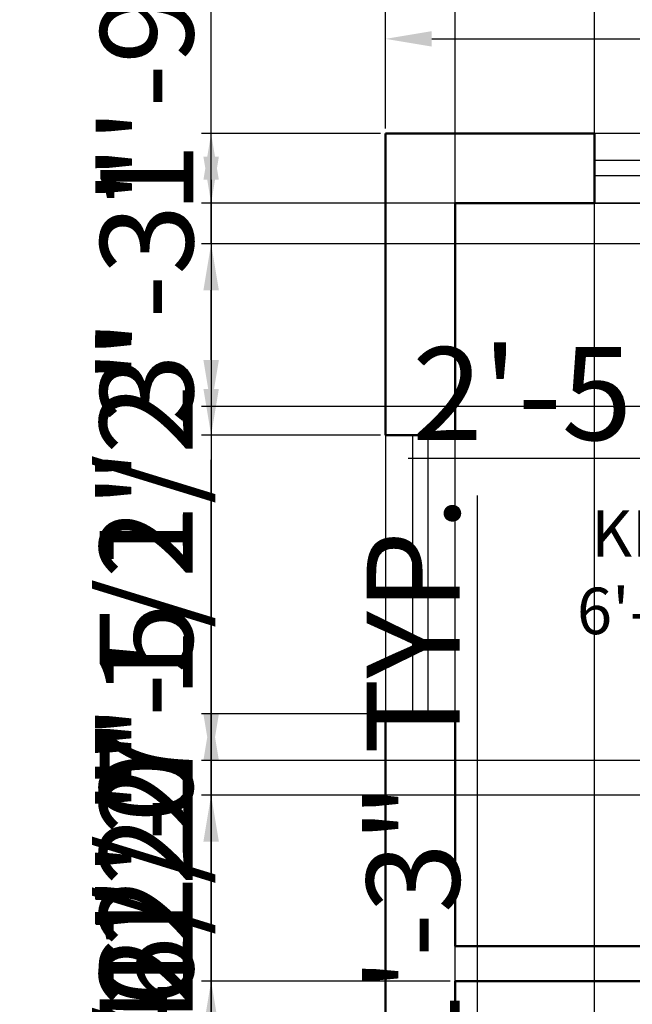
# Model space of a CAD drawing. Units: inches. Extents: x 1086 to 1501, y 383 to 973.
# Tile 4 of 7: x 1086 to 1165, y 723 to 850. Entities that reach past the tile are written whole.
import ezdxf

# ---------------------------------------------------------------- set-up
doc = ezdxf.new("R2010")
doc.units = ezdxf.units.IN
for name, color, linetype, lineweight in [('A-ANNO-DIMS', 2, 'Continuous', 18), ('A-AREA-IDEN', 7, 'Continuous', 25), ('wall', 7, 'Continuous', 50), ('window', 81, 'Continuous', 25)]:
    doc.layers.add(name, color=color, linetype=linetype, lineweight=lineweight)
doc.styles.get("Standard").update_dxf_attribs({"font": 'arial.ttf'})
doc.dimstyles.new('ISO-25', dxfattribs={"dimtxt": 12, "dimasz": 6, "dimexe": 1.25, "dimexo": 0.625, "dimtad": 1, "dimdec": 1, "dimlunit": 3, "dimtxsty": 'Standard', "dimcen": 2.5, "dimadec": 0, "dimazin": 0, "dimtfac": 1, "dimtdec": 1, "dimtmove": 0, "dimatfit": 3, "dimfxl": 1, "dimarcsym": 0})

# ---------------------------------------------------------------- blocks, each defined once
blk = doc.blocks.new('w1')
at = {"layer": 'window'}
for p, q in [((1475.33, 845.32), (1475.33, 809.32)), ((1477.33, 845.32), (1477.33, 809.32))]:
    blk.add_line(p, q, dxfattribs=at)
blk.add_lwpolyline([(1471.83, 809.32), (1480.83, 809.32), (1480.83, 845.32), (1471.83, 845.32)], close=True, dxfattribs=at)
blk = doc.blocks.new('*D9')
at = {"layer": 'A-ANNO-DIMS', "color": 0, "lineweight": -2, "transparency": 16777216}
for p, q in [((1133.43, 835.83), (1133.43, 848.67)), ((1403.43, 835.83), (1403.43, 848.67)), ((1139.43, 847.42), (1397.43, 847.42))]:
    blk.add_line(p, q, dxfattribs=at)
at = {"layer": 'A-ANNO-DIMS', "color": 0, "transparency": 16777216}
for points in [[(1139.43, 848.42), (1139.43, 846.42), (1133.43, 847.42)], [(1397.43, 848.42), (1397.43, 846.42), (1403.43, 847.42)]]:
    blk.add_solid(points, dxfattribs=at)
at = {"layer": 'Defpoints', "color": 0, "transparency": 16777216}
for p in [(1403.43, 847.42), (1133.43, 835.21), (1403.43, 835.21)]:
    blk.add_point(p, dxfattribs=at)
at = {"layer": 'A-ANNO-DIMS', "color": 0, "transparency": 16777216, "insert": (1268.43, 854.18), "char_height": 12, "attachment_point": 5}
blk.add_mtext('22\'-6"', dxfattribs=at)
blk = doc.blocks.new('*D18')
at = {"layer": 'A-ANNO-DIMS', "color": 0, "lineweight": -2, "transparency": 16777216}
for p, q in [((1244.93, 789.33), (1244.93, 794.46)), ((1274.43, 789.33), (1274.43, 794.46)), ((1244.93, 793.21), (1136.37, 793.21)), ((1268.43, 793.21), (1250.93, 793.21))]:
    blk.add_line(p, q, dxfattribs=at)
at = {"layer": 'A-ANNO-DIMS', "color": 0, "transparency": 16777216}
for points in [[(1250.93, 794.21), (1250.93, 792.21), (1244.93, 793.21)], [(1268.43, 794.21), (1268.43, 792.21), (1274.43, 793.21)]]:
    blk.add_solid(points, dxfattribs=at)
at = {"layer": 'Defpoints', "color": 0, "transparency": 16777216}
for p in [(1244.93, 793.21), (1244.93, 788.71), (1274.43, 788.71)]:
    blk.add_point(p, dxfattribs=at)
at = {"layer": 'A-ANNO-DIMS', "color": 0, "transparency": 16777216, "insert": (1187.65, 800.04), "char_height": 12, "attachment_point": 5}
blk.add_mtext('2\'-5 1/2" TYP.', dxfattribs=at)
blk = doc.blocks.new('*D25')
at = {"layer": 'A-ANNO-DIMS', "color": 0, "lineweight": -2, "transparency": 16777216}
for p, q in [((1147.7, 709.78), (1147.7, 712.78)), ((1163.51, 709.78), (1163.51, 712.78)), ((1153.7, 711.53), (1157.51, 711.53)), ((1163.51, 711.53), (1340.15, 711.53))]:
    blk.add_line(p, q, dxfattribs=at)
at = {"layer": 'A-ANNO-DIMS', "color": 0, "transparency": 16777216}
for points in [[(1153.7, 712.53), (1153.7, 710.53), (1147.7, 711.53)], [(1157.51, 712.53), (1157.51, 710.53), (1163.51, 711.53)]]:
    blk.add_solid(points, dxfattribs=at)
at = {"layer": 'Defpoints', "color": 0, "transparency": 16777216}
for p in [(1163.51, 711.53), (1147.7, 709.16), (1163.51, 709.16)]:
    blk.add_point(p, dxfattribs=at)
at = {"layer": 'A-ANNO-DIMS', "color": 0, "transparency": 16777216, "insert": (1254.83, 718.36), "char_height": 12, "attachment_point": 5}
blk.add_mtext('END CHAIR 1\'-4" TYP.', dxfattribs=at)
blk = doc.blocks.new('*D26')
at = {"layer": 'A-ANNO-DIMS', "color": 0, "lineweight": -2, "transparency": 16777216}
for p, q in [((1145.33, 709.16), (1145.33, 788.42)), ((1147.07, 709.16), (1144.08, 709.16)), ((1145.33, 700.13), (1145.33, 703.16)), ((1147.07, 694.13), (1144.08, 694.13))]:
    blk.add_line(p, q, dxfattribs=at)
at = {"layer": 'A-ANNO-DIMS', "color": 0, "transparency": 16777216}
for points in [[(1144.33, 703.16), (1146.33, 703.16), (1145.33, 709.16)], [(1144.33, 700.13), (1146.33, 700.13), (1145.33, 694.13)]]:
    blk.add_solid(points, dxfattribs=at)
at = {"layer": 'Defpoints', "color": 0, "transparency": 16777216}
for p in [(1145.33, 709.16), (1147.7, 709.16), (1147.7, 694.13)]:
    blk.add_point(p, dxfattribs=at)
at = {"layer": 'A-ANNO-DIMS', "color": 0, "transparency": 16777216, "insert": (1138.57, 751.79), "char_height": 12, "attachment_point": 5, "rotation": 90}
blk.add_mtext('1\'-3" TYP.', dxfattribs=at)
blk = doc.blocks.new('*D29')
at = {"layer": 'A-ANNO-DIMS', "color": 0, "lineweight": -2, "transparency": 16777216}
for p, q in [((1133.43, 835.83), (1133.43, 867.19)), ((1160.43, 835.83), (1160.43, 867.19)), ((1139.43, 865.94), (1154.43, 865.94)), ((1160.43, 865.94), (1199.78, 865.94))]:
    blk.add_line(p, q, dxfattribs=at)
at = {"layer": 'A-ANNO-DIMS', "color": 0, "transparency": 16777216}
for points in [[(1139.43, 866.94), (1139.43, 864.94), (1133.43, 865.94)], [(1154.43, 866.94), (1154.43, 864.94), (1160.43, 865.94)]]:
    blk.add_solid(points, dxfattribs=at)
at = {"layer": 'Defpoints', "color": 0, "transparency": 16777216}
for p in [(1160.43, 865.94), (1133.43, 835.21), (1160.43, 835.21)]:
    blk.add_point(p, dxfattribs=at)
at = {"layer": 'A-ANNO-DIMS', "color": 0, "transparency": 16777216, "insert": (1183.11, 872.7), "char_height": 12, "attachment_point": 5}
blk.add_mtext('2\'-3"', dxfattribs=at)
blk = doc.blocks.new('*D32')
at = {"layer": 'A-ANNO-DIMS', "color": 0, "lineweight": -2, "transparency": 16777216}
for p, q in [((1132.8, 835.21), (1109.68, 835.21)), ((1110.93, 829.21), (1110.93, 802.21)), ((1132.8, 796.21), (1109.68, 796.21))]:
    blk.add_line(p, q, dxfattribs=at)
at = {"layer": 'A-ANNO-DIMS', "color": 0, "transparency": 16777216}
for points in [[(1109.93, 829.21), (1111.93, 829.21), (1110.93, 835.21)], [(1109.93, 802.21), (1111.93, 802.21), (1110.93, 796.21)]]:
    blk.add_solid(points, dxfattribs=at)
at = {"layer": 'Defpoints', "color": 0, "transparency": 16777216}
for p in [(1133.43, 835.21), (1110.93, 796.21), (1133.43, 796.21)]:
    blk.add_point(p, dxfattribs=at)
at = {"layer": 'A-ANNO-DIMS', "color": 0, "transparency": 16777216, "insert": (1104.17, 815.71), "char_height": 12, "attachment_point": 5, "rotation": 90}
blk.add_mtext('3\'-3"', dxfattribs=at)
blk = doc.blocks.new('*D33')
at = {"layer": 'A-ANNO-DIMS', "color": 0, "lineweight": -2, "transparency": 16777216}
for p, q in [((1132.8, 760.21), (1109.68, 760.21)), ((1110.93, 754.21), (1110.93, 688.12)), ((1132.8, 682.12), (1109.68, 682.12))]:
    blk.add_line(p, q, dxfattribs=at)
at = {"layer": 'A-ANNO-DIMS', "color": 0, "transparency": 16777216}
for points in [[(1109.93, 754.21), (1111.93, 754.21), (1110.93, 760.21)], [(1109.93, 688.12), (1111.93, 688.12), (1110.93, 682.12)]]:
    blk.add_solid(points, dxfattribs=at)
at = {"layer": 'Defpoints', "color": 0, "transparency": 16777216}
for p in [(1133.43, 760.21), (1110.93, 682.12), (1133.43, 682.12)]:
    blk.add_point(p, dxfattribs=at)
at = {"layer": 'A-ANNO-DIMS', "color": 0, "transparency": 16777216, "insert": (1104.18, 721.16), "char_height": 12, "attachment_point": 5, "rotation": 90}
blk.add_mtext('6\'-6"', dxfattribs=at)
blk = doc.blocks.new('*D40')
at = {"layer": 'A-ANNO-DIMS', "color": 0, "lineweight": -2, "transparency": 16777216}
for p, q in [((1142.43, 502.33), (1142.43, 867.19)), ((1269.93, 502.33), (1269.93, 867.19)), ((1148.43, 865.94), (1263.93, 865.94))]:
    blk.add_line(p, q, dxfattribs=at)
at = {"layer": 'A-ANNO-DIMS', "color": 0, "transparency": 16777216}
for points in [[(1148.43, 866.94), (1148.43, 864.94), (1142.43, 865.94)], [(1263.93, 866.94), (1263.93, 864.94), (1269.93, 865.94)]]:
    blk.add_solid(points, dxfattribs=at)
at = {"layer": 'Defpoints', "color": 0, "transparency": 16777216}
for p in [(1269.93, 865.94), (1142.43, 501.71), (1269.93, 501.71)]:
    blk.add_point(p, dxfattribs=at)
at = {"layer": 'A-ANNO-DIMS', "color": 0, "transparency": 16777216, "insert": (1206.18, 872.77), "char_height": 12, "attachment_point": 5}
blk.add_mtext('10\'-7 1/2"', dxfattribs=at)
blk = doc.blocks.new('*D41')
at = {"layer": 'A-ANNO-DIMS', "color": 0, "lineweight": -2, "transparency": 16777216}
for p, q in [((1141.8, 725.71), (1109.68, 725.71)), ((1110.93, 507.71), (1110.93, 719.71)), ((1141.8, 501.71), (1109.68, 501.71))]:
    blk.add_line(p, q, dxfattribs=at)
at = {"layer": 'A-ANNO-DIMS', "color": 0, "transparency": 16777216}
for points in [[(1109.93, 719.71), (1111.93, 719.71), (1110.93, 725.71)], [(1109.93, 507.71), (1111.93, 507.71), (1110.93, 501.71)]]:
    blk.add_solid(points, dxfattribs=at)
at = {"layer": 'Defpoints', "color": 0, "transparency": 16777216}
for p in [(1110.93, 725.71), (1142.43, 725.71), (1142.43, 501.71)]:
    blk.add_point(p, dxfattribs=at)
at = {"layer": 'A-ANNO-DIMS', "color": 0, "transparency": 16777216, "insert": (1104.18, 613.71), "char_height": 12, "attachment_point": 5, "rotation": 90}
blk.add_mtext('18\'-8"', dxfattribs=at)
blk = doc.blocks.new('*D49')
at = {"layer": 'A-ANNO-DIMS', "color": 0, "lineweight": -2, "transparency": 16777216}
for p, q in [((1110.93, 760.21), (1110.93, 766.21)), ((1218.3, 754.21), (1109.68, 754.21)), ((1110.93, 754.21), (1110.93, 749.71)), ((1218.3, 749.71), (1109.68, 749.71)), ((1110.93, 743.71), (1110.93, 676.6))]:
    blk.add_line(p, q, dxfattribs=at)
at = {"layer": 'A-ANNO-DIMS', "color": 0, "transparency": 16777216}
for points in [[(1109.93, 760.21), (1111.93, 760.21), (1110.93, 754.21)], [(1109.93, 743.71), (1111.93, 743.71), (1110.93, 749.71)]]:
    blk.add_solid(points, dxfattribs=at)
at = {"layer": 'Defpoints', "color": 0, "transparency": 16777216}
for p in [(1218.93, 754.21), (1110.93, 749.71), (1218.93, 749.71)]:
    blk.add_point(p, dxfattribs=at)
at = {"layer": 'A-ANNO-DIMS', "color": 0, "transparency": 16777216, "insert": (1104.1, 707.15), "char_height": 12, "attachment_point": 5, "rotation": 90}
blk.add_mtext('0\'-4 1/2"', dxfattribs=at)
blk = doc.blocks.new('*D52')
at = {"layer": 'A-ANNO-DIMS', "color": 0, "lineweight": -2, "transparency": 16777216}
for p, q in [((1110.93, 692.71), (1110.93, 759.82)), ((1273.8, 686.71), (1109.68, 686.71)), ((1110.93, 682.21), (1110.93, 686.71)), ((1273.8, 682.21), (1109.68, 682.21)), ((1110.93, 676.21), (1110.93, 670.21))]:
    blk.add_line(p, q, dxfattribs=at)
at = {"layer": 'A-ANNO-DIMS', "color": 0, "transparency": 16777216}
for points in [[(1109.93, 692.71), (1111.93, 692.71), (1110.93, 686.71)], [(1109.93, 676.21), (1111.93, 676.21), (1110.93, 682.21)]]:
    blk.add_solid(points, dxfattribs=at)
at = {"layer": 'Defpoints', "color": 0, "transparency": 16777216}
for p in [(1110.93, 686.71), (1274.43, 686.71), (1274.43, 682.21)]:
    blk.add_point(p, dxfattribs=at)
at = {"layer": 'A-ANNO-DIMS', "color": 0, "transparency": 16777216, "insert": (1104.1, 729.26), "char_height": 12, "attachment_point": 5, "rotation": 90}
blk.add_mtext('0\'-4 1/2"', dxfattribs=at)
blk = doc.blocks.new('*D53')
at = {"layer": 'A-ANNO-DIMS', "color": 0, "lineweight": -2, "transparency": 16777216}
for p, q in [((1110.93, 686.71), (1110.93, 752.69)), ((1269.3, 686.71), (1109.68, 686.71)), ((1110.93, 679.21), (1110.93, 680.71)), ((1269.3, 673.21), (1109.68, 673.21))]:
    blk.add_line(p, q, dxfattribs=at)
at = {"layer": 'A-ANNO-DIMS', "color": 0, "transparency": 16777216}
for points in [[(1109.93, 680.71), (1111.93, 680.71), (1110.93, 686.71)], [(1109.93, 679.21), (1111.93, 679.21), (1110.93, 673.21)]]:
    blk.add_solid(points, dxfattribs=at)
at = {"layer": 'Defpoints', "color": 0, "transparency": 16777216}
for p in [(1110.93, 686.71), (1269.93, 686.71), (1269.93, 673.21)]:
    blk.add_point(p, dxfattribs=at)
at = {"layer": 'A-ANNO-DIMS', "color": 0, "transparency": 16777216, "insert": (1104.1, 722.7), "char_height": 12, "attachment_point": 5, "rotation": 90}
blk.add_mtext('1\'-1 1/2"', dxfattribs=at)
blk = doc.blocks.new('*D56')
at = {"layer": 'A-ANNO-DIMS', "color": 0, "lineweight": -2, "transparency": 16777216}
for p, q in [((1110.93, 832.21), (1110.93, 838.21)), ((1218.3, 826.21), (1109.68, 826.21)), ((1110.93, 826.21), (1110.93, 820.94)), ((1221.46, 820.94), (1109.68, 820.94)), ((1110.93, 814.94), (1110.93, 747.83))]:
    blk.add_line(p, q, dxfattribs=at)
at = {"layer": 'A-ANNO-DIMS', "color": 0, "transparency": 16777216}
for points in [[(1109.93, 832.21), (1111.93, 832.21), (1110.93, 826.21)], [(1109.93, 814.94), (1111.93, 814.94), (1110.93, 820.94)]]:
    blk.add_solid(points, dxfattribs=at)
at = {"layer": 'Defpoints', "color": 0, "transparency": 16777216}
for p in [(1218.93, 826.21), (1110.93, 820.94), (1222.08, 820.94)]:
    blk.add_point(p, dxfattribs=at)
at = {"layer": 'A-ANNO-DIMS', "color": 0, "transparency": 16777216, "insert": (1104.1, 778.39), "char_height": 12, "attachment_point": 5, "rotation": 90}
blk.add_mtext('0\'-5 1/2"', dxfattribs=at)
blk = doc.blocks.new('*D57')
at = {"layer": 'A-ANNO-DIMS', "color": 0, "lineweight": -2, "transparency": 16777216}
for p, q in [((1110.93, 820.94), (1110.93, 858.96)), ((1221.46, 820.94), (1109.68, 820.94)), ((1110.93, 805.94), (1110.93, 814.94)), ((1221.46, 799.94), (1109.68, 799.94))]:
    blk.add_line(p, q, dxfattribs=at)
at = {"layer": 'A-ANNO-DIMS', "color": 0, "transparency": 16777216}
for points in [[(1109.93, 814.94), (1111.93, 814.94), (1110.93, 820.94)], [(1109.93, 805.94), (1111.93, 805.94), (1110.93, 799.94)]]:
    blk.add_solid(points, dxfattribs=at)
at = {"layer": 'Defpoints', "color": 0, "transparency": 16777216}
for p in [(1110.93, 820.94), (1222.08, 820.94), (1222.08, 799.94)]:
    blk.add_point(p, dxfattribs=at)
at = {"layer": 'A-ANNO-DIMS', "color": 0, "transparency": 16777216, "insert": (1104.18, 842.95), "char_height": 12, "attachment_point": 5, "rotation": 90}
blk.add_mtext('1\'-9"', dxfattribs=at)
blk = doc.blocks.new('*D65')
at = {"layer": 'A-ANNO-DIMS', "color": 0, "lineweight": -2, "transparency": 16777216}
for p, q in [((1110.93, 725.71), (1110.93, 793.02)), ((1141.8, 725.71), (1109.68, 725.71)), ((1110.93, 700.13), (1110.93, 719.71)), ((1141.8, 694.13), (1109.68, 694.13))]:
    blk.add_line(p, q, dxfattribs=at)
at = {"layer": 'A-ANNO-DIMS', "color": 0, "transparency": 16777216}
for points in [[(1109.93, 719.71), (1111.93, 719.71), (1110.93, 725.71)], [(1109.93, 700.13), (1111.93, 700.13), (1110.93, 694.13)]]:
    blk.add_solid(points, dxfattribs=at)
at = {"layer": 'Defpoints', "color": 0, "transparency": 16777216}
for p in [(1110.93, 725.71), (1142.43, 725.71), (1142.43, 694.13)]:
    blk.add_point(p, dxfattribs=at)
at = {"layer": 'A-ANNO-DIMS', "color": 0, "transparency": 16777216, "insert": (1104.1, 762.36), "char_height": 12, "attachment_point": 5, "rotation": 90}
blk.add_mtext('2\'-7 1/2"', dxfattribs=at)
blk = doc.blocks.new('*D71')
at = {"layer": 'A-ANNO-DIMS', "color": 0, "lineweight": -2, "transparency": 16777216}
for p, q in [((1142.43, 589.29), (1142.43, 867.19)), ((1160.43, 589.29), (1160.43, 867.19)), ((1148.43, 865.94), (1154.43, 865.94)), ((1160.43, 865.94), (1198.45, 865.94))]:
    blk.add_line(p, q, dxfattribs=at)
at = {"layer": 'A-ANNO-DIMS', "color": 0, "transparency": 16777216}
for points in [[(1148.43, 866.94), (1148.43, 864.94), (1142.43, 865.94)], [(1154.43, 866.94), (1154.43, 864.94), (1160.43, 865.94)]]:
    blk.add_solid(points, dxfattribs=at)
at = {"layer": 'Defpoints', "color": 0, "transparency": 16777216}
for p in [(1160.43, 865.94), (1142.43, 588.67), (1160.43, 588.67)]:
    blk.add_point(p, dxfattribs=at)
at = {"layer": 'A-ANNO-DIMS', "color": 0, "transparency": 16777216, "insert": (1182.44, 872.69), "char_height": 12, "attachment_point": 5}
blk.add_mtext('1\'-6"', dxfattribs=at)

msp = doc.modelspace()

# ---------------------------------------------------------------- linework, layer by layer
at = {"layer": 'wall'}
for p, q in [((1133.43, 835.21), (1133.43, 796.21)), ((1160.43, 835.21), (1133.43, 835.21)), ((1160.43, 826.21), (1160.43, 835.21)), ((1142.43, 826.21), (1142.43, 796.21)), ((1160.43, 826.21), (1142.43, 826.21)), ((1142.43, 796.21), (1133.43, 796.21)), ((1142.43, 760.21), (1133.43, 760.21)), ((1133.43, 760.21), (1133.43, 682.12)), ((1142.43, 760.21), (1142.43, 730.21)), ((1214.43, 730.21), (1142.43, 730.21)), ((1218.93, 725.71), (1142.43, 725.71)), ((1142.43, 725.71), (1142.43, 682.12))]:
    msp.add_line(p, q, dxfattribs=at)

# ---------------------------------------------------------------- block references
at = {"layer": 'window', "rotation": 270}
msp.add_blockref('w1', (351.11, 2307.04), dxfattribs=at)
at = {"layer": 'window'}
msp.add_blockref('w1', (-338.4, -49.11), dxfattribs=at)

# ---------------------------------------------------------------- texts
at = {"layer": 'A-AREA-IDEN', "insert": (1158.17, 786.53), "char_height": 6, "attachment_point": 1}
msp.add_mtext_dynamic_manual_height_columns(' KITCHEN\\P6\'-0" X 8\'-0"', width=53.2651, gutter_width=12.5, heights=[0], dxfattribs=at)

# ---------------------------------------------------------------- dimensions: what is measured, and where the dimension line sits
at = {"layer": 'A-ANNO-DIMS'}
for base, p1, p2, override, picture, middle in [((1269.93, 865.94), (1142.43, 501.71), (1269.93, 501.71), {"dimdec": 1, "dimlfac": 1, "dimrnd": 0, "dimzin": 1, "dimdsep": 46, "dimlunit": 4, "dimfrac": 2}, '*D40', (1206.18, 872.77)), ((1160.43, 865.94), (1133.43, 835.21), (1160.43, 835.21), {"dimdec": 1, "dimlfac": 1, "dimrnd": 0, "dimzin": 1, "dimdsep": 46, "dimlunit": 4, "dimfrac": 2}, '*D29', (1183.11, 872.7)), ((1160.43, 865.94), (1142.43, 588.67), (1160.43, 588.67), {"dimdec": 1, "dimlfac": 1, "dimrnd": 0, "dimzin": 1, "dimdsep": 46, "dimlunit": 4, "dimfrac": 2}, '*D71', (1182.44, 872.69)), ((1403.43, 847.42), (1133.43, 835.21), (1403.43, 835.21), {"dimclrd": 0, "dimclre": 0, "dimclrt": 0}, '*D9', (1268.43, 854.18))]:
    dim = msp.add_linear_dim(base=base, p1=p1, p2=p2, dimstyle='ISO-25', override=override, dxfattribs=at)
    dim.commit()
    dim.dimension.update_dxf_attribs({"geometry": picture, "text_midpoint": middle})
for base, p1, p2, picture, middle in [((1110.93, 820.94), (1222.08, 799.94), (1222.08, 820.94), '*D57', (1104.18, 842.95)), ((1110.93, 820.94), (1218.93, 826.21), (1222.08, 820.94), '*D56', (1104.1, 778.39)), ((1110.93, 796.21), (1133.43, 835.21), (1133.43, 796.21), '*D32', (1104.17, 815.71)), ((1110.93, 725.71), (1142.43, 694.13), (1142.43, 725.71), '*D65', (1104.1, 762.36)), ((1110.93, 749.71), (1218.93, 754.21), (1218.93, 749.71), '*D49', (1104.1, 707.15)), ((1110.93, 686.71), (1274.43, 682.21), (1274.43, 686.71), '*D52', (1104.1, 729.26)), ((1110.93, 682.12), (1133.43, 760.21), (1133.43, 682.12), '*D33', (1104.18, 721.16)), ((1110.93, 686.71), (1269.93, 673.21), (1269.93, 686.71), '*D53', (1104.1, 722.7)), ((1110.93, 725.71), (1142.43, 501.71), (1142.43, 725.71), '*D41', (1104.18, 613.71))]:
    dim = msp.add_linear_dim(base=base, p1=p1, p2=p2, angle=90, dimstyle='ISO-25', override={"dimdec": 1, "dimlfac": 1, "dimrnd": 0, "dimzin": 1, "dimdsep": 46, "dimlunit": 4, "dimfrac": 2}, dxfattribs=at)
    dim.commit()
    dim.dimension.update_dxf_attribs({"geometry": picture, "text_midpoint": middle})
for base, p1, p2, angle, picture, middle in [((1244.93, 793.21), (1274.43, 788.71), (1244.93, 788.71), 180, '*D18', (1187.65, 800.04)), ((1145.33, 709.16), (1147.7, 694.13), (1147.7, 709.16), 90, '*D26', (1138.57, 751.79))]:
    dim = msp.add_linear_dim(base=base, p1=p1, p2=p2, angle=angle, text='<> TYP.', dimstyle='ISO-25', override={"dimdec": 1, "dimlfac": 1, "dimrnd": 0, "dimzin": 1, "dimdsep": 46, "dimlunit": 4, "dimfrac": 2}, dxfattribs=at)
    dim.commit()
    dim.dimension.update_dxf_attribs({"geometry": picture, "text_midpoint": middle})
dim = msp.add_linear_dim(base=(1163.51, 711.53), p1=(1147.7, 709.16), p2=(1163.51, 709.16), text='END CHAIR <> TYP.', dimstyle='ISO-25', override={"dimdec": 1, "dimlfac": 1, "dimrnd": 0, "dimzin": 1, "dimdsep": 46, "dimlunit": 4, "dimfrac": 2}, dxfattribs=at)
dim.commit()
dim.dimension.update_dxf_attribs({"geometry": '*D25', "text_midpoint": (1254.83, 718.36)})

doc.saveas('drawing.dxf')
